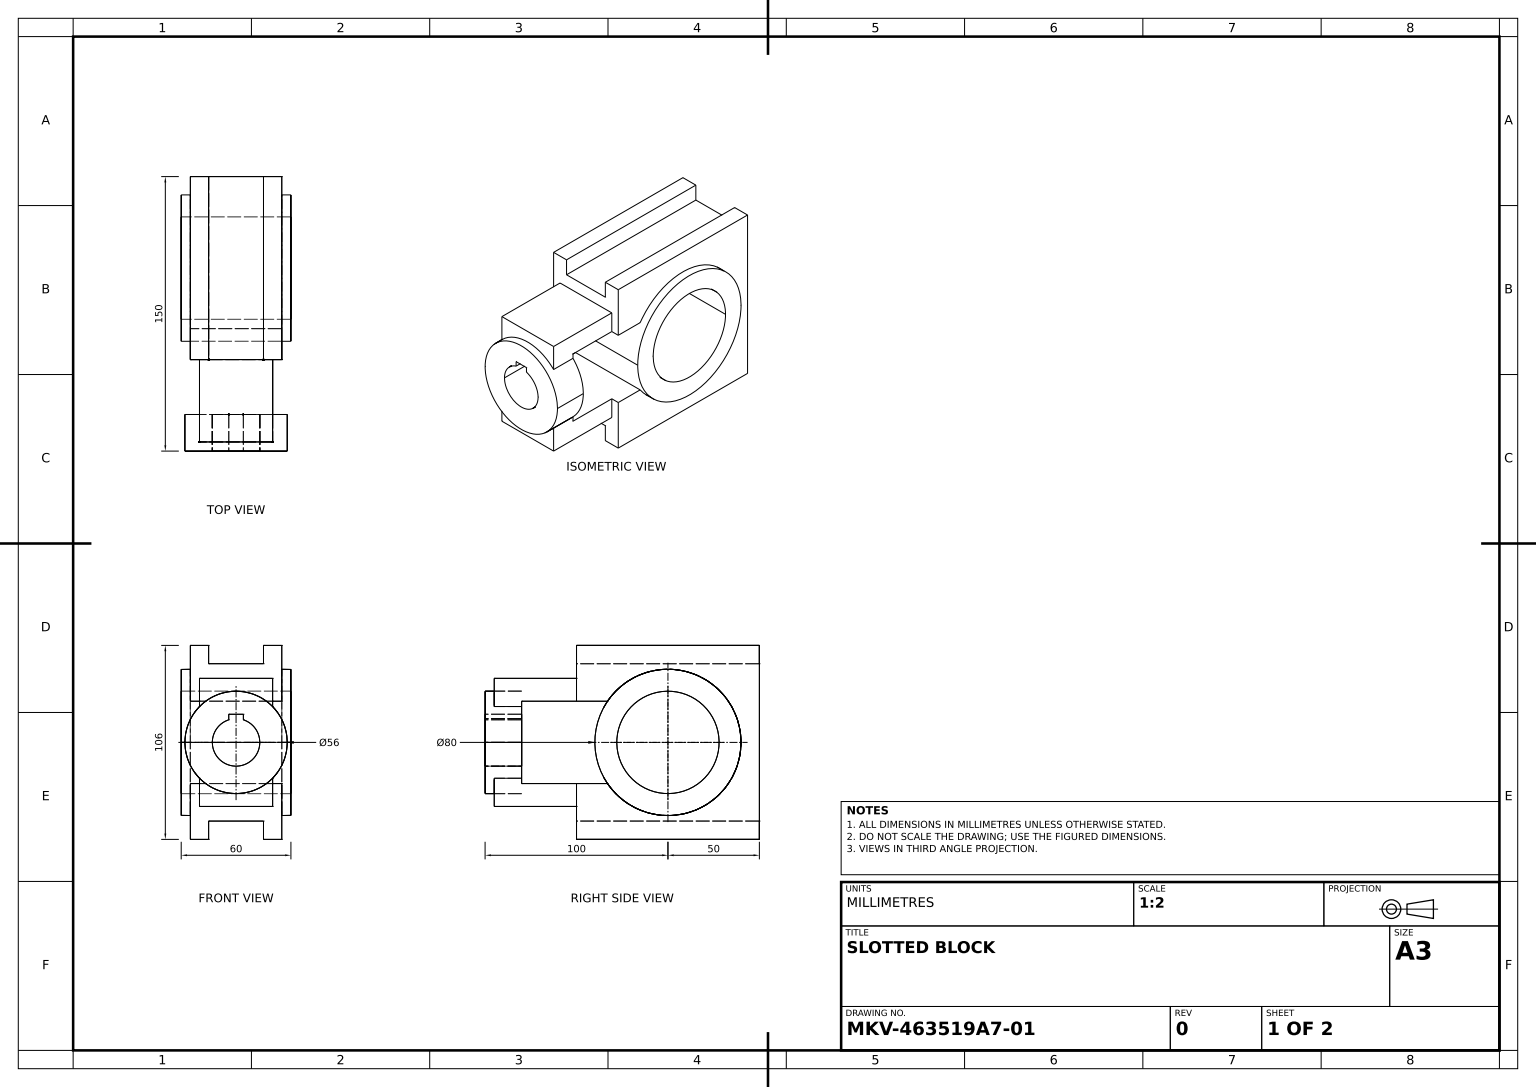
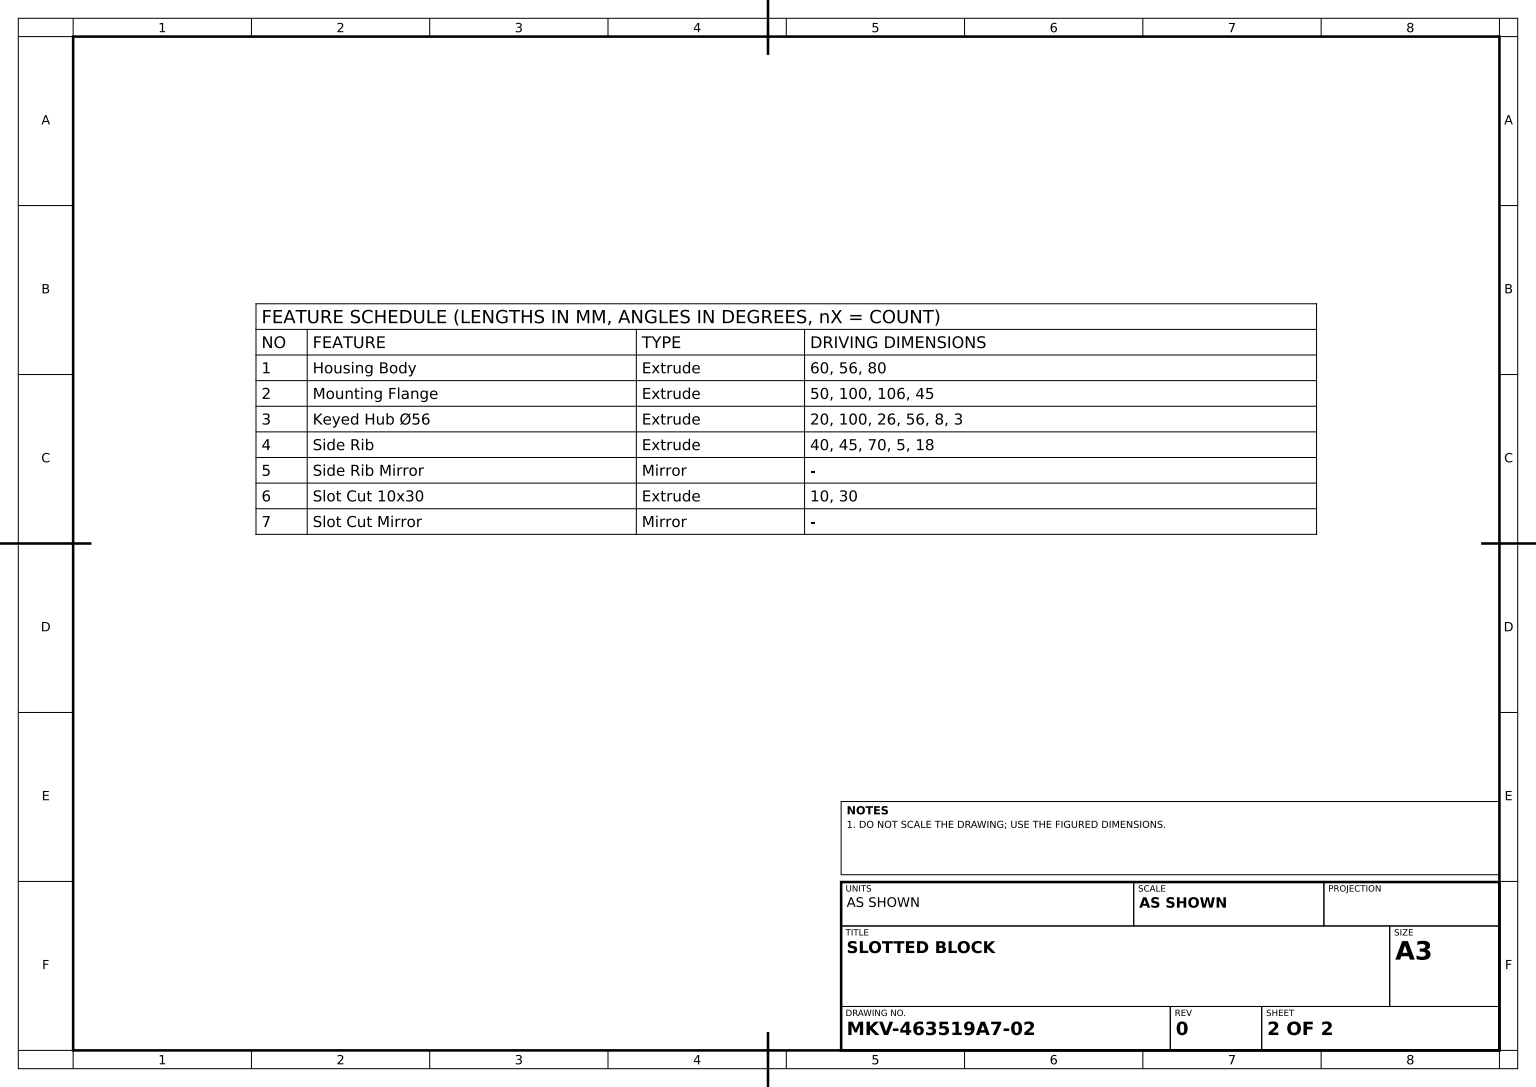
SolidWorks part; units mm, degrees
material "Plain Carbon Steel"
ref_plane "Front Plane" through (0, 0, 0) normal (0, 0, 1) x (1, 0, 0)
ref_plane "Top Plane" through (0, 0, 0) normal (0, 1, 0) x (1, 0, 0)
ref_plane "Right Plane" through (0, 0, 0) normal (1, 0, 0) x (0, 0, -1)
sketch "Housing Body Sketch" plane through (0, 0, 0) normal (1, 0, 0) x (0, 0, -1)
  circle A0 centre (0, 0) radius 28
  circle A1 centre (0, 0) radius 40
  dimension "D1" = 56
  dimension "D2" = 80
extrude "Housing Body" add sketch "Housing Body Sketch" along normal mid plane 60
sketch "Mounting Flange Sketch" plane through (0, 0, 0) normal (1, 0, 0) x (0, 0, -1)
  line L0 (-50, -22.5) -> (-50, -53)
  line L1 (-50, 53) -> (50, 53)
  line L2 (-50, 53) -> (-50, 22.5)
  line L3 (-50, -53) -> (50, -53)
  line L4 (50, 53) -> (50, -53)
  line L5 (-50, 53) -> (50, -53) construction
  line L6 (-50, -53) -> (50, 53) construction
  line L7 (-50, 22.5) -> (-33.0719, 22.5)
  line L9 (-50, -22.5) -> (-33.0719, -22.5)
  line L11 (0, 0) -> (-50, 0) construction
  circle A0 centre (0, 0) radius 40 construction
  circle A1 centre (0, 0) radius 40
  point P0 (0, 0)
  point P9 (-50, 0)
  dimension "D1" = 100
  dimension "D2" = 106
  dimension "D3" = 45
extrude "Mounting Flange" add sketch "Mounting Flange Sketch" along normal mid plane 50 contours A1 L9 L0 L3 L4 L1 L2 L7
sketch "Keyed Hub Sketch" plane through (0, 0, 0) normal (0, 0, 1) x (1, 0, 0)
  line L2 (-4, 12.3693) -> (-4, 15.3693)
  line L3 (-4, 15.3693) -> (4, 15.3693)
  line L4 (4, 12.3693) -> (4, 15.3693)
  circle A0 centre (0, 0) radius 28
  arc A1 (-4, 12.3693) -> (4, 12.3693) centre (0, 0) ccw
  point P8 (0, 15.3693)
  dimension "D1" = 26
  dimension "D2" = 56
  dimension "D3" = 8
  dimension "D4" = 3
extrude "Keyed Hub Ø56" add sketch "Keyed Hub Sketch" against normal blind 20 from offset 100 separate body
sketch "Side Rib Sketch" plane through (0, 0, 0) normal (1, 0, 0) x (0, 0, -1)
  line L0 (-50, 35) -> (-95, 35)
  line L1 (-50, 53) -> (-50, 22.5) construction
  line L2 (-95, 35) -> (-95, 17)
  line L3 (-95, 17) -> (-80, 17)
  line L4 (-80, -28) -> (-80, 28) construction
  line L5 (-80, 17) -> (-80, 22.5)
  line L6 (-80, 22.5) -> (-50, 22.5)
  line L7 (-50, 22.5) -> (-50, 35)
  line L8 (0, 0) -> (-80, 0) construction
  line L9 (-100, 28) -> (-100, -28) construction
  dimension "D1" = 45
  dimension "D2" = 70
  dimension "D3" = 5
  dimension "D4" = 18
extrude "Side Rib" add sketch "Side Rib Sketch" along normal mid plane 40
mirror "Side Rib Mirror" about plane through (0, 0, 0) normal (0, 1, 0) of "Side Rib"
sketch "Slot Cut Sketch" plane through (0, 0, 50) normal (0, 0, 1) x (1, 0, 0)
  line L0 (25, 53) -> (-25, 53) construction
  line L1 (-15, 53) -> (15, 53)
  line L2 (-15, 53) -> (-15, 43)
  line L3 (-15, 43) -> (15, 43)
  line L4 (15, 53) -> (15, 43)
  point P6 (0, 53)
  dimension "D1" = 10
  dimension "D2" = 30
extrude "Slot Cut 10x30" cut sketch "Slot Cut Sketch" against normal through all
mirror "Slot Cut Mirror" about plane through (0, 0, 0) normal (0, 1, 0) of "Slot Cut 10x30"
